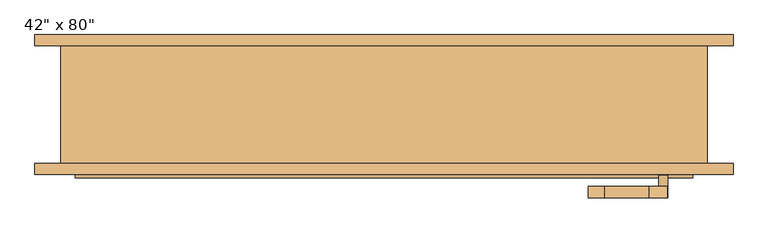
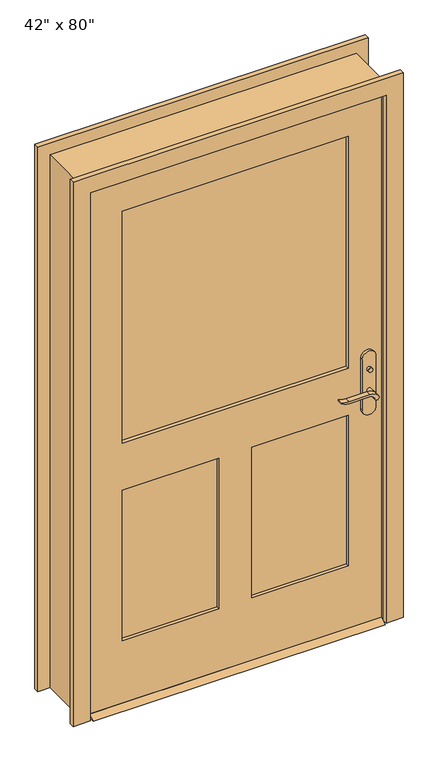
"""IFC4 building model written with IfcOpenShell, lengths in millimetres: door geometry."""

from ifc_helpers import new_model, si_unit, point, frame, frame_2d, origin, place, context, project, spatial, polyline, circle_curve, trimmed, segment, composite_curve, outline, extrude, faceted_brep, source, transform, mapped, element, save


def door_374e07cf(model_context):
    return source(origin(), model_context, "Body", "SolidModel", [
        extrude(outline(polyline([(-63.5, 12.7), (-38.1, 0.0), (-123.825, 0.0), (-98.425, 12.7), (-63.5, 12.7)])), frame((-533.4, 0.0, 0.0), z_axis=(1.0, 0.0, 0.0), x_axis=(0.0, 1.0, 0.0)), (0.0, 0.0, 1.0), 1066.8),
        extrude(outline(polyline([(487.6, -43.5), (487.6, -53.5), (477.6, -53.5), (477.6, -43.5), (487.6, -43.5)])), frame((0.0, 0.0, 981.9), z_axis=(0.0, 0.0, 1.0), x_axis=(1.0, 0.0, 0.0)), (0.0, 0.0, 1.0), 30.0),
        extrude(outline(composite_curve([segment(trimmed(circle_curve(frame_2d((996.9, 482.6)), 8.0), [point((996.9, 474.6))], [point((996.9, 490.6))], False, "CARTESIAN"), True, "CONTINUOUS"), segment(trimmed(circle_curve(frame_2d((996.9, 482.6)), 8.0), [point((996.9, 490.6))], [point((996.9, 474.6))], False, "CARTESIAN"), True, "CONTINUOUS")], self_intersect=False)), frame((0.0, -118.425, 0.0), z_axis=(0.0, 1.0, 0.0), x_axis=(0.0, 0.0, 1.0)), (0.0, 0.0, 1.0), 10.0),
        extrude(outline(composite_curve([segment(trimmed(circle_curve(frame_2d((897.1555521, 458.9324871)), 37.2832219), [point((919.0523287, 489.1081363))], [point((934.4, 457.2325667))], False, "CARTESIAN"), True, "CONTINUOUS"), segment(polyline([(934.4, 457.2325667), (934.4, 380.9564091)]), True, "CONTINUOUS"), segment(trimmed(circle_curve(frame_2d((1017.6850638, 381.0227909)), 83.2850902), [point((934.4, 380.9564091))], [point((939.4, 352.6))], True, "CARTESIAN"), True, "CONTINUOUS"), segment(polyline([(939.4, 352.6), (936.6135558, 352.6)]), True, "CONTINUOUS"), segment(trimmed(circle_curve(frame_2d((986.6709207, 384.5396612)), 59.3791355), [point((936.6135558, 352.6))], [point((927.4, 380.9564091))], False, "CARTESIAN"), True, "CONTINUOUS"), segment(polyline([(927.4, 380.9564091), (927.4, 457.2138099)]), True, "CONTINUOUS"), segment(trimmed(circle_curve(frame_2d((909.2738613, 457.2138099)), 18.1261387), [point((927.4, 457.2138099))], [point((914.4, 474.6))], True, "CARTESIAN"), True, "CONTINUOUS"), segment(trimmed(circle_curve(frame_2d((914.4, 482.6)), 8.0), [point((914.4, 474.6))], [point((919.0523287, 489.1081363))], False, "CARTESIAN"), True, "CONTINUOUS")], self_intersect=False)), frame((0.0, -23.5, 0.0), z_axis=(0.0, 1.0, 0.0), x_axis=(0.0, 0.0, 1.0)), (0.0, 0.0, 1.0), 20.0),
        extrude(outline(composite_curve([segment(trimmed(circle_curve(frame_2d((914.4, 482.6)), 8.0), [point((914.3999903, 474.6))], [point((919.0523287, 489.1081363))], False, "CARTESIAN"), True, "CONTINUOUS"), segment(trimmed(circle_curve(frame_2d((897.1555521, 458.9324871)), 37.2832219), [point((919.0523287, 489.1081363))], [point((934.4, 457.2325667))], False, "CARTESIAN"), True, "CONTINUOUS"), segment(polyline([(934.4, 457.2325667), (934.4, 380.9564091)]), True, "CONTINUOUS"), segment(trimmed(circle_curve(frame_2d((1017.6850638, 381.0227909)), 83.2850902), [point((934.4, 380.9564091))], [point((939.4, 352.6))], True, "CARTESIAN"), True, "CONTINUOUS"), segment(polyline([(939.4, 352.6), (936.6135558, 352.6)]), True, "CONTINUOUS"), segment(trimmed(circle_curve(frame_2d((986.6709207, 384.5396612)), 59.3791355), [point((936.6135558, 352.6))], [point((927.4, 380.9564091))], False, "CARTESIAN"), True, "CONTINUOUS"), segment(polyline([(927.4, 380.9564091), (927.4, 457.2138122)]), True, "CONTINUOUS"), segment(trimmed(circle_curve(frame_2d((909.2738682, 457.2138122)), 18.1261318), [point((927.4, 457.2138122))], [point((914.3999903, 474.6))], True, "CARTESIAN"), True, "CONTINUOUS")], self_intersect=False)), frame((0.0, -158.425, 0.0), z_axis=(0.0, 1.0, 0.0), x_axis=(0.0, 0.0, 1.0)), (0.0, 0.0, 1.0), 20.0),
        extrude(outline(composite_curve([segment(trimmed(circle_curve(frame_2d((914.4, 482.6)), 8.0), [point((914.4, 474.6))], [point((914.4, 490.6))], False, "CARTESIAN"), True, "CONTINUOUS"), segment(trimmed(circle_curve(frame_2d((914.4, 482.6)), 8.0), [point((914.4, 490.6))], [point((914.4, 474.6))], False, "CARTESIAN"), True, "CONTINUOUS")], self_intersect=False)), frame((0.0, -53.5, 0.0), z_axis=(0.0, 1.0, 0.0), x_axis=(0.0, 0.0, 1.0)), (0.0, 0.0, 1.0), 30.0),
        extrude(outline(composite_curve([segment(trimmed(circle_curve(frame_2d((914.4, 482.6)), 8.0), [point((914.4, 474.6))], [point((914.4, 490.6))], False, "CARTESIAN"), True, "CONTINUOUS"), segment(trimmed(circle_curve(frame_2d((914.4, 482.6)), 8.0), [point((914.4, 490.6))], [point((914.4, 474.6))], False, "CARTESIAN"), True, "CONTINUOUS")], self_intersect=False)), frame((0.0, -138.425, 0.0), z_axis=(0.0, 1.0, 0.0), x_axis=(0.0, 0.0, 1.0)), (0.0, 0.0, 1.0), 30.0),
        extrude(outline(composite_curve([segment(polyline([(844.4, 507.6), (1039.4, 507.6)]), True, "CONTINUOUS"), segment(trimmed(circle_curve(frame_2d((1039.4, 482.6)), 25.0), [point((1039.4, 507.6))], [point((1039.4, 457.6))], False, "CARTESIAN"), True, "CONTINUOUS"), segment(polyline([(1039.4, 457.6), (844.4, 457.6)]), True, "CONTINUOUS"), segment(trimmed(circle_curve(frame_2d((844.4, 482.6)), 25.0), [point((844.4, 457.6))], [point((844.4, 507.6))], False, "CARTESIAN"), True, "CONTINUOUS")], self_intersect=False)), frame((0.0, -63.5, 0.0), z_axis=(0.0, 1.0, 0.0), x_axis=(0.0, 0.0, 1.0)), (0.0, 0.0, 1.0), 10.0),
        extrude(outline(composite_curve([segment(polyline([(844.4, 507.6), (1039.4, 507.6)]), True, "CONTINUOUS"), segment(trimmed(circle_curve(frame_2d((1039.4, 482.6)), 25.0), [point((1039.4, 507.6))], [point((1039.4, 457.6))], False, "CARTESIAN"), True, "CONTINUOUS"), segment(polyline([(1039.4, 457.6), (844.4, 457.6)]), True, "CONTINUOUS"), segment(trimmed(circle_curve(frame_2d((844.4, 482.6)), 25.0), [point((844.4, 457.6))], [point((844.4, 507.6))], False, "CARTESIAN"), True, "CONTINUOUS")], self_intersect=False)), frame((0.0, -108.425, 0.0), z_axis=(0.0, 1.0, 0.0), x_axis=(0.0, 0.0, 1.0)), (0.0, 0.0, 1.0), 10.0),
        extrude(outline(polyline([(2032.0, -533.4), (12.7, -533.4), (12.7, 533.4), (2032.0, 533.4), (2032.0, -533.4)]), holes=[polyline([(1016.0, -412.75), (1911.35, -412.75), (1911.35, 412.75), (1016.0, 412.75), (1016.0, -412.75)]), polyline([(835.025, -60.325), (254.0, -60.325), (254.0, -412.75), (835.025, -412.75), (835.025, -60.325)]), polyline([(835.025, 412.75), (254.0, 412.75), (254.0, 60.325), (835.025, 60.325), (835.025, 412.75)])]), frame((0.0, -98.425, 0.0), z_axis=(0.0, 1.0, 0.0), x_axis=(0.0, 0.0, 1.0)), (0.0, 0.0, 1.0), 34.925),
        faceted_brep([(558.8, -98.425, 0.0), (533.4, -98.425, 0.0), (533.4, -63.5, 0.0), (520.7, -63.5, 0.0), (520.7, -28.575, 0.0), (533.4, -28.575, 0.0), (533.4, 104.775, 0.0), (558.8, 104.775, 0.0), (558.8, 104.775, 2057.4), (558.8, -98.425, 2057.4), (533.4, 104.775, 2032.0), (-533.4, 104.775, 2032.0), (-533.4, 104.775, 0.0), (-558.8, 104.775, 0.0), (-558.8, 104.775, 2057.4), (533.4, -28.575, 2032.0), (520.7, -28.575, 2019.3), (-520.7, -28.575, 2019.3), (-520.7, -28.575, 0.0), (-533.4, -28.575, 0.0), (-533.4, -28.575, 2032.0), (520.7, -63.5, 2019.3), (533.4, -63.5, 2032.0), (-533.4, -63.5, 2032.0), (-533.4, -63.5, 0.0), (-520.7, -63.5, 0.0), (-520.7, -63.5, 2019.3), (533.4, -98.425, 2032.0), (-558.8, -98.425, 2057.4), (-558.8, -98.425, 0.0), (-533.4, -98.425, 0.0), (-533.4, -98.425, 2032.0)], [[[0, 1, 2, 3, 4, 5, 6, 7]], [[7, 8, 9, 0]], [[6, 10, 11, 12, 13, 14, 8, 7]], [[5, 15, 10, 6]], [[4, 16, 17, 18, 19, 20, 15, 5]], [[3, 21, 16, 4]], [[2, 22, 23, 24, 25, 26, 21, 3]], [[1, 27, 22, 2]], [[0, 9, 28, 29, 30, 31, 27, 1]], [[8, 14, 28, 9]], [[15, 20, 11, 10]], [[21, 26, 17, 16]], [[27, 31, 23, 22]], [[29, 13, 12, 19, 18, 25, 24, 30]], [[14, 13, 29, 28]], [[20, 19, 12, 11]], [[26, 25, 18, 17]], [[31, 30, 24, 23]]]),
        extrude(outline(polyline([(-60.325, -75.1416667), (-60.325, -86.7833333), (-412.75, -86.7833333), (-412.75, -75.1416667), (-60.325, -75.1416667)])), frame((0.0, 0.0, 254.0), z_axis=(0.0, 0.0, 1.0), x_axis=(1.0, 0.0, 0.0)), (0.0, 0.0, 1.0), 581.025),
        extrude(outline(polyline([(412.75, -75.1416667), (412.75, -86.7833333), (60.325, -86.7833333), (60.325, -75.1416667), (412.75, -75.1416667)])), frame((0.0, 0.0, 254.0), z_axis=(0.0, 0.0, 1.0), x_axis=(1.0, 0.0, 0.0)), (0.0, 0.0, 1.0), 581.025),
        extrude(outline(polyline([(412.75, -77.47), (412.75, -84.455), (-412.75, -84.455), (-412.75, -77.47), (412.75, -77.47)])), frame((0.0, 0.0, 1016.0), z_axis=(0.0, 0.0, 1.0), x_axis=(1.0, 0.0, 0.0)), (0.0, 0.0, 1.0), 895.35),
        extrude(outline(polyline([(0.0, -539.75), (2038.35, -539.75), (2038.35, 539.75), (0.0, 539.75), (0.0, 603.25), (2101.85, 603.25), (2101.85, -603.25), (0.0, -603.25), (0.0, -539.75)])), frame((0.0, 104.775, 0.0), z_axis=(0.0, 1.0, 0.0), x_axis=(0.0, 0.0, 1.0)), (0.0, 0.0, 1.0), 19.05),
        extrude(outline(polyline([(0.0, -539.75), (2038.35, -539.75), (2038.35, 539.75), (0.0, 539.75), (0.0, 603.25), (2101.85, 603.25), (2101.85, -603.25), (0.0, -603.25), (0.0, -539.75)])), frame((0.0, -117.475, 0.0), z_axis=(0.0, 1.0, 0.0), x_axis=(0.0, 0.0, 1.0)), (0.0, 0.0, 1.0), 19.05),
    ])


if __name__ == "__main__":
    model = new_model("IFC4")
    model_context = context("Model", 3, world=origin())
    ifc_project = project(units=[si_unit("LENGTHUNIT", "METRE", prefix="MILLI")], contexts=[model_context])
    site = spatial("IfcSite", under=ifc_project)
    building = spatial("IfcBuilding", under=site)
    placement = place(None, origin())
    door_shape = door_374e07cf(model_context)
    element("IfcDoor", 1, ObjectType="42\" x 80\"", at=placement, inside=building, context=model_context, shape_type="MappedRepresentation", body=[
        mapped(door_shape, transform((0.0, 0.0, 0.0), x_axis=(1.0, 0.0, 0.0), y_axis=(0.0, 1.0, 0.0), z_axis=(0.0, 0.0, 1.0))),
    ])
    save(model, "model.ifc")

# Revit data of these elements
# Type "42\" x 80\""
#   Type Mark = "8"
#   Assembly Code = "B2030100"
#   Analytic Construction = "French door, wood frame with single glass"
#   Top Rail = 0' - 4 3/4"
#   Threshold Offset [instance default] = 0' - 0 1/2"
#   Thickness = 0' - 1 3/8"
#   Thermal Resistance (R) = 1.0696 (h·ft²·°F)/BTU
#   Swing Angle [instance default] = 90.00°
#   Stiles = 0' - 4 3/4"
#   Rough Width = 3' - 8"
#   Rough Height = 6' - 9"
#   Lock Rail = 0' - 7 1/8"
#   Height = 6' - 8"
#   Width = 3' - 6"
#   Heat Transfer Coefficient (U) = 0.9350 BTU/(h·ft²·°F)
#   Door Offset [instance default] = 0' - 0"
#   Bottom Rail = 0' - 9 1/2"
#   Threshold [instance default] = yes
#   Function = 1
#   Exterior Trim [instance default] = yes
#   Trim Material = Cherry
#   Threshold Material = Cherry
#   Panel Material = Cherry
#   Glazing = Glass
#   Frame Material = Cherry
#   Door Handle Material = Aluminum
#   Visual Light Transmittance = 0
#   Solar Heat Gain Coefficient = 0
#   Wall Closure = (empty or 0)
#   Construction Type = (empty or 0)
# Element 1 (IfcDoor, "42\" x 80\"")
#   Materials on its faces: "Cherry", "Aluminum", "Glass"
# Materials
#   "Cherry": class "Wood", colour RGB 226 177 128, transparency 0, Description = "Prunus Serotina", Cost = 0
#   "Glass": class "Glass", colour RGB 0 128 192, transparency 0.75, Description = "Soda Lime Glass", Cost = 0
#   "Aluminum": class "Metal", colour RGB 247 247 247, transparency 0, Description = "Aluminum 6061", Cost = 0
